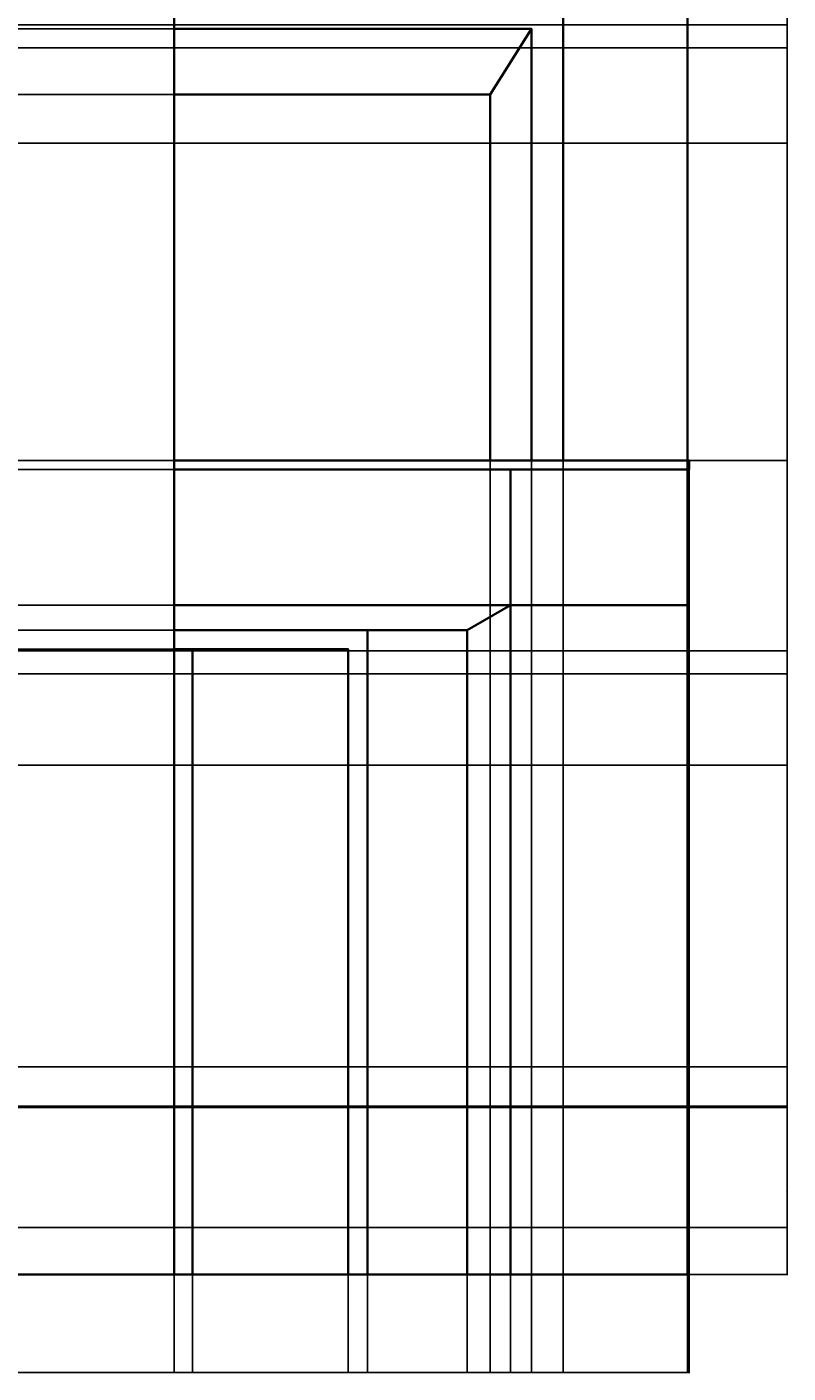
# Model space of a CAD drawing. Units: feet. Extents: x 4092 to 5585, y 725 to 1390.
# Tile 6 of 7: x 5346 to 5585, y 725 to 1146. Entities that reach past the tile are written whole.
import ezdxf

# ---------------------------------------------------------------- set-up
doc = ezdxf.new("R2010")
doc.units = ezdxf.units.FT
doc.layers.add('A-ANNO-DIMS', color=2, linetype='Continuous', lineweight=18)
doc.layers.add('A-ELEV', color=7, linetype='Continuous', lineweight=35)
doc.styles.get("Standard").update_dxf_attribs({"font": 'arial.ttf'})
doc.dimstyles.get("Standard").update_dxf_attribs({"dimtxt": 0.18, "dimasz": 0.18, "dimexe": 0.18, "dimexo": 0.0625, "dimgap": 0.09, "dimtad": 0, "dimtih": 1, "dimtoh": 1, "dimdec": 1, "dimzin": 0, "dimdsep": 46, "dimlunit": 3, "dimtxsty": 'Standard', "dimcen": 0.09, "dimadec": 0, "dimazin": 0, "dimtfac": 1, "dimtdec": 1, "dimtofl": 0, "dimtmove": 0, "dimatfit": 3, "dimfxl": 1, "dimtolj": 1, "dimtzin": 0, "dimarcsym": 0})

# ---------------------------------------------------------------- blocks, each defined once
blk = doc.blocks.new('*D4')
at = {"layer": 'A-ANNO-DIMS', "color": 0, "lineweight": -2, "transparency": 16777216}
for p, q in [((4953.29, 755.89), (4953.29, 725.07)), ((5553.29, 755.89), (5553.29, 725.07)), ((4953.47, 725.25), (5253, 725.25)), ((5553.11, 725.25), (5253.58, 725.25))]:
    blk.add_line(p, q, dxfattribs=at)
at = {"layer": 'A-ANNO-DIMS', "color": 0, "transparency": 16777216}
for points in [[(4953.47, 725.28), (4953.47, 725.22), (4953.29, 725.25)], [(5553.11, 725.28), (5553.11, 725.22), (5553.29, 725.25)]]:
    blk.add_solid(points, dxfattribs=at)
at = {"layer": 'Defpoints', "color": 0, "transparency": 16777216}
for p in [(4953.29, 755.95), (5553.29, 755.95), (5553.29, 725.25)]:
    blk.add_point(p, dxfattribs=at)
at = {"layer": 'A-ANNO-DIMS', "color": 0, "transparency": 16777216, "insert": (5253.29, 725.25), "char_height": 0.18, "attachment_point": 5}
blk.add_mtext('\\A1;600', dxfattribs=at)
blk = doc.blocks.new('*D5')
at = {"layer": 'A-ANNO-DIMS', "color": 0, "lineweight": -2, "transparency": 16777216}
for p, q in [((5264.26, 1358.97), (5584.71, 1358.97)), ((5584.53, 1358.79), (5584.53, 1057.64)), ((5584.53, 756.13), (5584.53, 1057.28)), ((5553.36, 755.95), (5584.71, 755.95))]:
    blk.add_line(p, q, dxfattribs=at)
at = {"layer": 'A-ANNO-DIMS', "color": 0, "transparency": 16777216}
for points in [[(5584.5, 1358.79), (5584.56, 1358.79), (5584.53, 1358.97)], [(5584.5, 756.13), (5584.56, 756.13), (5584.53, 755.95)]]:
    blk.add_solid(points, dxfattribs=at)
at = {"layer": 'Defpoints', "color": 0, "transparency": 16777216}
for p in [(5264.2, 1358.97), (5584.53, 1358.97), (5553.29, 755.95)]:
    blk.add_point(p, dxfattribs=at)
at = {"layer": 'A-ANNO-DIMS', "color": 0, "transparency": 16777216, "insert": (5584.53, 1057.46), "char_height": 0.18, "attachment_point": 5}
blk.add_mtext('\\A1;603', dxfattribs=at)
blk = doc.blocks.new('*D33')
at = {"layer": 'A-ANNO-DIMS', "color": 0, "lineweight": -2, "transparency": 16777216}
for p, q in [((5153.4, 808.21), (5584.71, 808.21)), ((5584.53, 808.03), (5584.53, 782.26)), ((5584.53, 756.13), (5584.53, 781.9)), ((5153.4, 755.95), (5584.71, 755.95))]:
    blk.add_line(p, q, dxfattribs=at)
at = {"layer": 'A-ANNO-DIMS', "color": 0, "transparency": 16777216}
for points in [[(5584.5, 808.03), (5584.56, 808.03), (5584.53, 808.21)], [(5584.5, 756.13), (5584.56, 756.13), (5584.53, 755.95)]]:
    blk.add_solid(points, dxfattribs=at)
at = {"layer": 'Defpoints', "color": 0, "transparency": 16777216}
for p in [(5153.34, 808.21), (5584.53, 808.21), (5153.34, 755.95)]:
    blk.add_point(p, dxfattribs=at)
at = {"layer": 'A-ANNO-DIMS', "color": 0, "transparency": 16777216, "insert": (5584.53, 782.08), "char_height": 0.18, "attachment_point": 5}
blk.add_mtext('\\A1;52.27', dxfattribs=at)
blk = doc.blocks.new('*D34')
at = {"layer": 'A-ANNO-DIMS', "color": 0, "lineweight": -2, "transparency": 16777216}
for p, q in [((5153.4, 915.42), (5584.71, 915.42)), ((5584.53, 915.24), (5584.53, 862)), ((5584.53, 808.39), (5584.53, 861.63)), ((5153.4, 808.21), (5584.71, 808.21))]:
    blk.add_line(p, q, dxfattribs=at)
at = {"layer": 'A-ANNO-DIMS', "color": 0, "transparency": 16777216}
for points in [[(5584.5, 915.24), (5584.56, 915.24), (5584.53, 915.42)], [(5584.5, 808.39), (5584.56, 808.39), (5584.53, 808.21)]]:
    blk.add_solid(points, dxfattribs=at)
at = {"layer": 'Defpoints', "color": 0, "transparency": 16777216}
for p in [(5153.34, 915.42), (5584.53, 915.42), (5153.34, 808.21)]:
    blk.add_point(p, dxfattribs=at)
at = {"layer": 'A-ANNO-DIMS', "color": 0, "transparency": 16777216, "insert": (5584.53, 861.82), "char_height": 0.18, "attachment_point": 5}
blk.add_mtext('\\A1;107.2', dxfattribs=at)
blk = doc.blocks.new('*D35')
at = {"layer": 'A-ANNO-DIMS', "color": 0, "lineweight": -2, "transparency": 16777216}
for p, q in [((5153.4, 944.01), (5584.71, 944.01)), ((5584.53, 943.83), (5584.53, 929.9)), ((5584.53, 915.6), (5584.53, 929.53)), ((5153.4, 915.42), (5584.71, 915.42))]:
    blk.add_line(p, q, dxfattribs=at)
at = {"layer": 'A-ANNO-DIMS', "color": 0, "transparency": 16777216}
for points in [[(5584.5, 943.83), (5584.56, 943.83), (5584.53, 944.01)], [(5584.5, 915.6), (5584.56, 915.6), (5584.53, 915.42)]]:
    blk.add_solid(points, dxfattribs=at)
at = {"layer": 'Defpoints', "color": 0, "transparency": 16777216}
for p in [(5153.34, 944.01), (5584.53, 944.01), (5153.34, 915.42)]:
    blk.add_point(p, dxfattribs=at)
at = {"layer": 'A-ANNO-DIMS', "color": 0, "transparency": 16777216, "insert": (5584.53, 929.71), "char_height": 0.18, "attachment_point": 5}
blk.add_mtext('\\A1;28.59', dxfattribs=at)
blk = doc.blocks.new('*D36')
at = {"layer": 'A-ANNO-DIMS', "color": 0, "lineweight": -2, "transparency": 16777216}
for p, q in [((5160.6, 951.2), (5584.71, 951.2)), ((5584.53, 951.02), (5584.53, 947.79)), ((5153.4, 944.01), (5584.71, 944.01)), ((5584.53, 944.19), (5584.53, 947.42))]:
    blk.add_line(p, q, dxfattribs=at)
at = {"layer": 'A-ANNO-DIMS', "color": 0, "transparency": 16777216}
for points in [[(5584.5, 951.02), (5584.56, 951.02), (5584.53, 951.2)], [(5584.5, 944.19), (5584.56, 944.19), (5584.53, 944.01)]]:
    blk.add_solid(points, dxfattribs=at)
at = {"layer": 'Defpoints', "color": 0, "transparency": 16777216}
for p in [(5160.53, 951.2), (5584.53, 951.2), (5153.34, 944.01)]:
    blk.add_point(p, dxfattribs=at)
at = {"layer": 'A-ANNO-DIMS', "color": 0, "transparency": 16777216, "insert": (5584.53, 947.61), "char_height": 0.18, "attachment_point": 5}
blk.add_mtext('\\A1;7.194', dxfattribs=at)
blk = doc.blocks.new('*D37')
at = {"layer": 'A-ANNO-DIMS', "color": 0, "lineweight": -2, "transparency": 16777216}
for p, q in [((5094.36, 770.68), (5584.71, 770.68)), ((5584.53, 770.5), (5584.53, 763.5)), ((5584.53, 756.13), (5584.53, 763.13)), ((5057.45, 755.95), (5584.71, 755.95))]:
    blk.add_line(p, q, dxfattribs=at)
at = {"layer": 'A-ANNO-DIMS', "color": 0, "transparency": 16777216}
for points in [[(5584.5, 770.5), (5584.56, 770.5), (5584.53, 770.68)], [(5584.5, 756.13), (5584.56, 756.13), (5584.53, 755.95)]]:
    blk.add_solid(points, dxfattribs=at)
at = {"layer": 'Defpoints', "color": 0, "transparency": 16777216}
for p in [(5094.3, 770.68), (5584.53, 770.68), (5057.39, 755.95)]:
    blk.add_point(p, dxfattribs=at)
at = {"layer": 'A-ANNO-DIMS', "color": 0, "transparency": 16777216, "insert": (5584.53, 763.31), "char_height": 0.18, "attachment_point": 5}
blk.add_mtext('\\A1;14.73', dxfattribs=at)
blk = doc.blocks.new('*D38')
at = {"layer": 'A-ANNO-DIMS', "color": 0, "lineweight": -2, "transparency": 16777216}
for p, q in [((5094.36, 808.65), (5584.71, 808.65)), ((5584.53, 808.47), (5584.53, 789.85)), ((5584.53, 770.86), (5584.53, 789.48)), ((5094.36, 770.68), (5584.71, 770.68))]:
    blk.add_line(p, q, dxfattribs=at)
at = {"layer": 'A-ANNO-DIMS', "color": 0, "transparency": 16777216}
for points in [[(5584.5, 808.47), (5584.56, 808.47), (5584.53, 808.65)], [(5584.5, 770.86), (5584.56, 770.86), (5584.53, 770.68)]]:
    blk.add_solid(points, dxfattribs=at)
at = {"layer": 'Defpoints', "color": 0, "transparency": 16777216}
for p in [(5094.3, 808.65), (5584.53, 808.65), (5094.3, 770.68)]:
    blk.add_point(p, dxfattribs=at)
at = {"layer": 'A-ANNO-DIMS', "color": 0, "transparency": 16777216, "insert": (5584.53, 789.67), "char_height": 0.18, "attachment_point": 5}
blk.add_mtext('\\A1;37.97', dxfattribs=at)
blk = doc.blocks.new('*D57')
at = {"layer": 'A-ANNO-DIMS', "color": 0, "lineweight": -2, "transparency": 16777216}
for p, q in [((5153.4, 1110.12), (5584.71, 1110.12)), ((5584.53, 1109.94), (5584.53, 1060.64)), ((5584.53, 1010.97), (5584.53, 1060.27)), ((5185.39, 1010.79), (5584.71, 1010.79))]:
    blk.add_line(p, q, dxfattribs=at)
at = {"layer": 'A-ANNO-DIMS', "color": 0, "transparency": 16777216}
for points in [[(5584.5, 1109.94), (5584.56, 1109.94), (5584.53, 1110.12)], [(5584.5, 1010.97), (5584.56, 1010.97), (5584.53, 1010.79)]]:
    blk.add_solid(points, dxfattribs=at)
at = {"layer": 'Defpoints', "color": 0, "transparency": 16777216}
for p in [(5153.34, 1110.12), (5584.53, 1110.12), (5185.33, 1010.79)]:
    blk.add_point(p, dxfattribs=at)
at = {"layer": 'A-ANNO-DIMS', "color": 0, "transparency": 16777216, "insert": (5584.53, 1060.45), "char_height": 0.18, "attachment_point": 5}
blk.add_mtext('\\A1;99.33', dxfattribs=at)
blk = doc.blocks.new('*D58')
at = {"layer": 'A-ANNO-DIMS', "color": 0, "lineweight": -2, "transparency": 16777216}
for p, q in [((5153.4, 1139.88), (5584.71, 1139.88)), ((5584.53, 1139.7), (5584.53, 1125.18)), ((5584.53, 1110.3), (5584.53, 1124.82)), ((5153.4, 1110.12), (5584.71, 1110.12))]:
    blk.add_line(p, q, dxfattribs=at)
at = {"layer": 'A-ANNO-DIMS', "color": 0, "transparency": 16777216}
for points in [[(5584.5, 1139.7), (5584.56, 1139.7), (5584.53, 1139.88)], [(5584.5, 1110.3), (5584.56, 1110.3), (5584.53, 1110.12)]]:
    blk.add_solid(points, dxfattribs=at)
at = {"layer": 'Defpoints', "color": 0, "transparency": 16777216}
for p in [(5153.34, 1139.88), (5584.53, 1139.88), (5153.34, 1110.12)]:
    blk.add_point(p, dxfattribs=at)
at = {"layer": 'A-ANNO-DIMS', "color": 0, "transparency": 16777216, "insert": (5584.53, 1125), "char_height": 0.18, "attachment_point": 5}
blk.add_mtext('\\A1;29.76', dxfattribs=at)
blk = doc.blocks.new('*D59')
at = {"layer": 'A-ANNO-DIMS', "color": 0, "lineweight": -2, "transparency": 16777216}
for p, q in [((5185.39, 1147.07), (5584.71, 1147.07)), ((5584.53, 1146.89), (5584.53, 1143.66)), ((5584.53, 1140.06), (5584.53, 1143.3)), ((5153.4, 1139.88), (5584.71, 1139.88))]:
    blk.add_line(p, q, dxfattribs=at)
at = {"layer": 'A-ANNO-DIMS', "color": 0, "transparency": 16777216}
for points in [[(5584.5, 1146.89), (5584.56, 1146.89), (5584.53, 1147.07)], [(5584.5, 1140.06), (5584.56, 1140.06), (5584.53, 1139.88)]]:
    blk.add_solid(points, dxfattribs=at)
at = {"layer": 'Defpoints', "color": 0, "transparency": 16777216}
for p in [(5185.33, 1147.07), (5584.53, 1147.07), (5153.34, 1139.88)]:
    blk.add_point(p, dxfattribs=at)
at = {"layer": 'A-ANNO-DIMS', "color": 0, "transparency": 16777216, "insert": (5584.53, 1143.48), "char_height": 0.18, "attachment_point": 5}
blk.add_mtext('\\A1;7.194', dxfattribs=at)
blk = doc.blocks.new('*D64')
at = {"layer": 'A-ANNO-DIMS', "color": 0, "lineweight": -2, "transparency": 16777216}
for p, q in [((5285.79, 755.89), (5285.79, 725.07)), ((5392.55, 755.89), (5392.55, 725.07)), ((5285.97, 725.25), (5338.72, 725.25)), ((5392.37, 725.25), (5339.63, 725.25))]:
    blk.add_line(p, q, dxfattribs=at)
at = {"layer": 'A-ANNO-DIMS', "color": 0, "transparency": 16777216}
for points in [[(5285.97, 725.28), (5285.97, 725.22), (5285.79, 725.25)], [(5392.37, 725.28), (5392.37, 725.22), (5392.55, 725.25)]]:
    blk.add_solid(points, dxfattribs=at)
at = {"layer": 'Defpoints', "color": 0, "transparency": 16777216}
for p in [(5285.79, 755.95), (5392.55, 755.95), (5392.55, 725.25)]:
    blk.add_point(p, dxfattribs=at)
at = {"layer": 'A-ANNO-DIMS', "color": 0, "transparency": 16777216, "insert": (5339.17, 725.25), "char_height": 0.18, "attachment_point": 5}
blk.add_mtext('\\A1;106.76', dxfattribs=at)
blk = doc.blocks.new('*D65')
at = {"layer": 'A-ANNO-DIMS', "color": 0, "lineweight": -2, "transparency": 16777216}
for p, q in [((5392.55, 755.89), (5392.55, 725.07)), ((5398.25, 755.89), (5398.25, 725.07)), ((5392.73, 725.25), (5395.01, 725.25)), ((5398.07, 725.25), (5395.79, 725.25))]:
    blk.add_line(p, q, dxfattribs=at)
at = {"layer": 'A-ANNO-DIMS', "color": 0, "transparency": 16777216}
for points in [[(5392.73, 725.28), (5392.73, 725.22), (5392.55, 725.25)], [(5398.07, 725.28), (5398.07, 725.22), (5398.25, 725.25)]]:
    blk.add_solid(points, dxfattribs=at)
at = {"layer": 'Defpoints', "color": 0, "transparency": 16777216}
for p in [(5392.55, 755.95), (5398.25, 755.95), (5398.25, 725.25)]:
    blk.add_point(p, dxfattribs=at)
at = {"layer": 'A-ANNO-DIMS', "color": 0, "transparency": 16777216, "insert": (5395.4, 725.25), "char_height": 0.18, "attachment_point": 5}
blk.add_mtext('\\A1;5.694', dxfattribs=at)
blk = doc.blocks.new('*D66')
at = {"layer": 'A-ANNO-DIMS', "color": 0, "lineweight": -2, "transparency": 16777216}
for p, q in [((5398.25, 755.89), (5398.25, 725.07)), ((5447.06, 755.89), (5447.06, 725.07)), ((5398.43, 725.25), (5422.27, 725.25)), ((5446.88, 725.25), (5423.03, 725.25))]:
    blk.add_line(p, q, dxfattribs=at)
at = {"layer": 'A-ANNO-DIMS', "color": 0, "transparency": 16777216}
for points in [[(5398.43, 725.28), (5398.43, 725.22), (5398.25, 725.25)], [(5446.88, 725.28), (5446.88, 725.22), (5447.06, 725.25)]]:
    blk.add_solid(points, dxfattribs=at)
at = {"layer": 'Defpoints', "color": 0, "transparency": 16777216}
for p in [(5398.25, 755.95), (5447.06, 755.95), (5447.06, 725.25)]:
    blk.add_point(p, dxfattribs=at)
at = {"layer": 'A-ANNO-DIMS', "color": 0, "transparency": 16777216, "insert": (5422.65, 725.25), "char_height": 0.18, "attachment_point": 5}
blk.add_mtext('\\A1;48.81', dxfattribs=at)
blk = doc.blocks.new('*D67')
at = {"layer": 'A-ANNO-DIMS', "color": 0, "lineweight": -2, "transparency": 16777216}
for p, q in [((5447.06, 755.89), (5447.06, 725.07)), ((5453.06, 755.89), (5453.06, 725.07)), ((5447.24, 725.25), (5449.91, 725.25)), ((5452.88, 725.25), (5450.21, 725.25))]:
    blk.add_line(p, q, dxfattribs=at)
at = {"layer": 'A-ANNO-DIMS', "color": 0, "transparency": 16777216}
for points in [[(5447.24, 725.28), (5447.24, 725.22), (5447.06, 725.25)], [(5452.88, 725.28), (5452.88, 725.22), (5453.06, 725.25)]]:
    blk.add_solid(points, dxfattribs=at)
at = {"layer": 'Defpoints', "color": 0, "transparency": 16777216}
for p in [(5447.06, 755.95), (5453.06, 755.95), (5453.06, 725.25)]:
    blk.add_point(p, dxfattribs=at)
at = {"layer": 'A-ANNO-DIMS', "color": 0, "transparency": 16777216, "insert": (5450.06, 725.25), "char_height": 0.18, "attachment_point": 5}
blk.add_mtext('\\A1;6', dxfattribs=at)
blk = doc.blocks.new('*D68')
at = {"layer": 'A-ANNO-DIMS', "color": 0, "lineweight": -2, "transparency": 16777216}
for p, q in [((5453.06, 755.89), (5453.06, 725.07)), ((5484.32, 755.89), (5484.32, 725.07)), ((5453.24, 725.25), (5468.29, 725.25)), ((5484.14, 725.25), (5469.08, 725.25))]:
    blk.add_line(p, q, dxfattribs=at)
at = {"layer": 'A-ANNO-DIMS', "color": 0, "transparency": 16777216}
for points in [[(5453.24, 725.28), (5453.24, 725.22), (5453.06, 725.25)], [(5484.14, 725.28), (5484.14, 725.22), (5484.32, 725.25)]]:
    blk.add_solid(points, dxfattribs=at)
at = {"layer": 'Defpoints', "color": 0, "transparency": 16777216}
for p in [(5453.06, 755.95), (5484.32, 755.95), (5484.32, 725.25)]:
    blk.add_point(p, dxfattribs=at)
at = {"layer": 'A-ANNO-DIMS', "color": 0, "transparency": 16777216, "insert": (5468.69, 725.25), "char_height": 0.18, "attachment_point": 5}
blk.add_mtext('\\A1;31.26', dxfattribs=at)
blk = doc.blocks.new('*D69')
at = {"layer": 'A-ANNO-DIMS', "color": 0, "lineweight": -2, "transparency": 16777216}
for p, q in [((5484.32, 755.89), (5484.32, 725.07)), ((5497.93, 755.89), (5497.93, 725.07)), ((5484.5, 725.25), (5490.76, 725.25)), ((5497.75, 725.25), (5491.49, 725.25))]:
    blk.add_line(p, q, dxfattribs=at)
at = {"layer": 'A-ANNO-DIMS', "color": 0, "transparency": 16777216}
for points in [[(5484.5, 725.28), (5484.5, 725.22), (5484.32, 725.25)], [(5497.75, 725.28), (5497.75, 725.22), (5497.93, 725.25)]]:
    blk.add_solid(points, dxfattribs=at)
at = {"layer": 'Defpoints', "color": 0, "transparency": 16777216}
for p in [(5484.32, 755.95), (5497.93, 755.95), (5497.93, 725.25)]:
    blk.add_point(p, dxfattribs=at)
at = {"layer": 'A-ANNO-DIMS', "color": 0, "transparency": 16777216, "insert": (5491.12, 725.25), "char_height": 0.18, "attachment_point": 5}
blk.add_mtext('\\A1;13.61', dxfattribs=at)
blk = doc.blocks.new('*D70')
at = {"layer": 'A-ANNO-DIMS', "color": 0, "lineweight": -2, "transparency": 16777216}
for p, q in [((5497.93, 755.89), (5497.93, 725.07)), ((5553.29, 755.89), (5553.29, 725.07)), ((5498.11, 725.25), (5525.22, 725.25)), ((5553.11, 725.25), (5526, 725.25))]:
    blk.add_line(p, q, dxfattribs=at)
at = {"layer": 'A-ANNO-DIMS', "color": 0, "transparency": 16777216}
for points in [[(5498.11, 725.28), (5498.11, 725.22), (5497.93, 725.25)], [(5553.11, 725.28), (5553.11, 725.22), (5553.29, 725.25)]]:
    blk.add_solid(points, dxfattribs=at)
at = {"layer": 'Defpoints', "color": 0, "transparency": 16777216}
for p in [(5497.93, 755.95), (5553.29, 755.95), (5553.29, 725.25)]:
    blk.add_point(p, dxfattribs=at)
at = {"layer": 'A-ANNO-DIMS', "color": 0, "transparency": 16777216, "insert": (5525.61, 725.25), "char_height": 0.18, "attachment_point": 5}
blk.add_mtext('\\A1;55.36', dxfattribs=at)
blk = doc.blocks.new('*D73')
at = {"layer": 'A-ANNO-DIMS', "color": 0, "lineweight": -2, "transparency": 16777216}
for p, q in [((5339.81, 820.92), (5584.71, 820.92)), ((5584.53, 820.74), (5584.53, 788.62)), ((5584.53, 756.13), (5584.53, 788.25)), ((5285.85, 755.95), (5584.71, 755.95))]:
    blk.add_line(p, q, dxfattribs=at)
at = {"layer": 'A-ANNO-DIMS', "color": 0, "transparency": 16777216}
for points in [[(5584.5, 820.74), (5584.56, 820.74), (5584.53, 820.92)], [(5584.5, 756.13), (5584.56, 756.13), (5584.53, 755.95)]]:
    blk.add_solid(points, dxfattribs=at)
at = {"layer": 'Defpoints', "color": 0, "transparency": 16777216}
for p in [(5339.75, 820.92), (5584.53, 820.92), (5285.79, 755.95)]:
    blk.add_point(p, dxfattribs=at)
at = {"layer": 'A-ANNO-DIMS', "color": 0, "transparency": 16777216, "insert": (5584.53, 788.43), "char_height": 0.18, "attachment_point": 5}
blk.add_mtext('\\A1;64.97', dxfattribs=at)
blk = doc.blocks.new('*D75')
at = {"layer": 'A-ANNO-DIMS', "color": 0, "lineweight": -2, "transparency": 16777216}
for p, q in [((5392.49, 951.65), (4921.27, 951.65)), ((4921.45, 951.47), (4921.45, 853.98)), ((4921.45, 756.13), (4921.45, 853.62)), ((5392.49, 755.95), (4921.27, 755.95))]:
    blk.add_line(p, q, dxfattribs=at)
at = {"layer": 'A-ANNO-DIMS', "color": 0, "transparency": 16777216}
for points in [[(4921.42, 951.47), (4921.48, 951.47), (4921.45, 951.65)], [(4921.42, 756.13), (4921.48, 756.13), (4921.45, 755.95)]]:
    blk.add_solid(points, dxfattribs=at)
at = {"layer": 'Defpoints', "color": 0, "transparency": 16777216}
for p in [(4921.45, 951.65), (5392.55, 951.65), (5392.55, 755.95)]:
    blk.add_point(p, dxfattribs=at)
at = {"layer": 'A-ANNO-DIMS', "color": 0, "transparency": 16777216, "insert": (4921.45, 853.8), "char_height": 0.18, "attachment_point": 5}
blk.add_mtext('\\A1;195.7', dxfattribs=at)
blk = doc.blocks.new('*D76')
at = {"layer": 'A-ANNO-DIMS', "color": 0, "lineweight": -2, "transparency": 16777216}
for p, q in [((5392.49, 957.65), (4921.27, 957.65)), ((4921.45, 957.47), (4921.45, 954.83)), ((4921.45, 951.83), (4921.45, 954.46)), ((5392.49, 951.65), (4921.27, 951.65))]:
    blk.add_line(p, q, dxfattribs=at)
at = {"layer": 'A-ANNO-DIMS', "color": 0, "transparency": 16777216}
for points in [[(4921.42, 957.47), (4921.48, 957.47), (4921.45, 957.65)], [(4921.42, 951.83), (4921.48, 951.83), (4921.45, 951.65)]]:
    blk.add_solid(points, dxfattribs=at)
at = {"layer": 'Defpoints', "color": 0, "transparency": 16777216}
for p in [(4921.45, 957.65), (5392.55, 957.65), (5392.55, 951.65)]:
    blk.add_point(p, dxfattribs=at)
at = {"layer": 'A-ANNO-DIMS', "color": 0, "transparency": 16777216, "insert": (4921.45, 954.65), "char_height": 0.18, "attachment_point": 5}
blk.add_mtext('\\A1;6', dxfattribs=at)
blk = doc.blocks.new('*D77')
at = {"layer": 'A-ANNO-DIMS', "color": 0, "lineweight": -2, "transparency": 16777216}
for p, q in [((5392.49, 965.48), (4921.27, 965.48)), ((4921.45, 965.3), (4921.45, 961.74)), ((4921.45, 957.83), (4921.45, 961.38)), ((5392.49, 957.65), (4921.27, 957.65))]:
    blk.add_line(p, q, dxfattribs=at)
at = {"layer": 'A-ANNO-DIMS', "color": 0, "transparency": 16777216}
for points in [[(4921.42, 965.3), (4921.48, 965.3), (4921.45, 965.48)], [(4921.42, 957.83), (4921.48, 957.83), (4921.45, 957.65)]]:
    blk.add_solid(points, dxfattribs=at)
at = {"layer": 'Defpoints', "color": 0, "transparency": 16777216}
for p in [(4921.45, 965.48), (5392.55, 965.48), (5392.55, 957.65)]:
    blk.add_point(p, dxfattribs=at)
at = {"layer": 'A-ANNO-DIMS', "color": 0, "transparency": 16777216, "insert": (4921.45, 961.56), "char_height": 0.18, "attachment_point": 5}
blk.add_mtext('\\A1;7.833', dxfattribs=at)
blk = doc.blocks.new('*D78')
at = {"layer": 'A-ANNO-DIMS', "color": 0, "lineweight": -2, "transparency": 16777216}
for p, q in [((5392.49, 1007.95), (4921.27, 1007.95)), ((4921.45, 1007.77), (4921.45, 986.89)), ((4921.45, 965.66), (4921.45, 986.53)), ((5392.49, 965.48), (4921.27, 965.48))]:
    blk.add_line(p, q, dxfattribs=at)
at = {"layer": 'A-ANNO-DIMS', "color": 0, "transparency": 16777216}
for points in [[(4921.42, 1007.77), (4921.48, 1007.77), (4921.45, 1007.95)], [(4921.42, 965.66), (4921.48, 965.66), (4921.45, 965.48)]]:
    blk.add_solid(points, dxfattribs=at)
at = {"layer": 'Defpoints', "color": 0, "transparency": 16777216}
for p in [(4921.45, 1007.95), (5392.55, 1007.95), (5392.55, 965.48)]:
    blk.add_point(p, dxfattribs=at)
at = {"layer": 'A-ANNO-DIMS', "color": 0, "transparency": 16777216, "insert": (4921.45, 986.71), "char_height": 0.18, "attachment_point": 5}
blk.add_mtext('\\A1;42.47', dxfattribs=at)
blk = doc.blocks.new('*D79')
at = {"layer": 'A-ANNO-DIMS', "color": 0, "lineweight": -2, "transparency": 16777216}
for p, q in [((5392.49, 1125.34), (4921.27, 1125.34)), ((4921.45, 1125.16), (4921.45, 1068.25)), ((4921.45, 1010.97), (4921.45, 1067.88)), ((5392.49, 1010.79), (4921.27, 1010.79))]:
    blk.add_line(p, q, dxfattribs=at)
at = {"layer": 'A-ANNO-DIMS', "color": 0, "transparency": 16777216}
for points in [[(4921.42, 1125.16), (4921.48, 1125.16), (4921.45, 1125.34)], [(4921.42, 1010.97), (4921.48, 1010.97), (4921.45, 1010.79)]]:
    blk.add_solid(points, dxfattribs=at)
at = {"layer": 'Defpoints', "color": 0, "transparency": 16777216}
for p in [(4921.45, 1125.34), (5392.55, 1125.34), (5392.55, 1010.79)]:
    blk.add_point(p, dxfattribs=at)
at = {"layer": 'A-ANNO-DIMS', "color": 0, "transparency": 16777216, "insert": (4921.45, 1068.07), "char_height": 0.18, "attachment_point": 5}
blk.add_mtext('\\A1;114.55', dxfattribs=at)
blk = doc.blocks.new('*D80')
at = {"layer": 'A-ANNO-DIMS', "color": 0, "lineweight": -2, "transparency": 16777216}
for p, q in [((5392.49, 1145.86), (4921.27, 1145.86)), ((4921.45, 1145.68), (4921.45, 1135.78)), ((4921.45, 1125.52), (4921.45, 1135.42)), ((5392.49, 1125.34), (4921.27, 1125.34))]:
    blk.add_line(p, q, dxfattribs=at)
at = {"layer": 'A-ANNO-DIMS', "color": 0, "transparency": 16777216}
for points in [[(4921.42, 1145.68), (4921.48, 1145.68), (4921.45, 1145.86)], [(4921.42, 1125.52), (4921.48, 1125.52), (4921.45, 1125.34)]]:
    blk.add_solid(points, dxfattribs=at)
at = {"layer": 'Defpoints', "color": 0, "transparency": 16777216}
for p in [(4921.45, 1145.86), (5392.55, 1145.86), (5392.55, 1125.34)]:
    blk.add_point(p, dxfattribs=at)
at = {"layer": 'A-ANNO-DIMS', "color": 0, "transparency": 16777216, "insert": (4921.45, 1135.6), "char_height": 0.18, "attachment_point": 5}
blk.add_mtext('\\A1;20.52', dxfattribs=at)
blk = doc.blocks.new('*D81')
at = {"layer": 'A-ANNO-DIMS', "color": 0, "lineweight": -2, "transparency": 16777216}
for p, q in [((5392.49, 1171.51), (4921.27, 1171.51)), ((4921.45, 1171.33), (4921.45, 1158.87)), ((4921.45, 1146.04), (4921.45, 1158.5)), ((5392.49, 1145.86), (4921.27, 1145.86))]:
    blk.add_line(p, q, dxfattribs=at)
at = {"layer": 'A-ANNO-DIMS', "color": 0, "transparency": 16777216}
for points in [[(4921.42, 1171.33), (4921.48, 1171.33), (4921.45, 1171.51)], [(4921.42, 1146.04), (4921.48, 1146.04), (4921.45, 1145.86)]]:
    blk.add_solid(points, dxfattribs=at)
at = {"layer": 'Defpoints', "color": 0, "transparency": 16777216}
for p in [(4921.45, 1171.51), (5392.55, 1171.51), (5392.55, 1145.86)]:
    blk.add_point(p, dxfattribs=at)
at = {"layer": 'A-ANNO-DIMS', "color": 0, "transparency": 16777216, "insert": (4921.45, 1158.69), "char_height": 0.18, "attachment_point": 5}
blk.add_mtext('\\A1;25.65', dxfattribs=at)
blk = doc.blocks.new('*D88')
at = {"layer": 'A-ANNO-DIMS', "color": 0, "lineweight": -2, "transparency": 16777216}
for p, q in [((5392.55, 1010.73), (5392.55, 725.07)), ((5491.48, 1010.73), (5491.48, 725.07)), ((5392.73, 725.25), (5441.62, 725.25)), ((5491.3, 725.25), (5442.41, 725.25))]:
    blk.add_line(p, q, dxfattribs=at)
at = {"layer": 'A-ANNO-DIMS', "color": 0, "transparency": 16777216}
for points in [[(5392.73, 725.28), (5392.73, 725.22), (5392.55, 725.25)], [(5491.3, 725.28), (5491.3, 725.22), (5491.48, 725.25)]]:
    blk.add_solid(points, dxfattribs=at)
at = {"layer": 'Defpoints', "color": 0, "transparency": 16777216}
for p in [(5392.55, 1010.79), (5491.48, 1010.79), (5491.48, 725.25)]:
    blk.add_point(p, dxfattribs=at)
at = {"layer": 'A-ANNO-DIMS', "color": 0, "transparency": 16777216, "insert": (5442.01, 725.25), "char_height": 0.18, "attachment_point": 5}
blk.add_mtext('\\A1;98.93', dxfattribs=at)
blk = doc.blocks.new('*D89')
at = {"layer": 'A-ANNO-DIMS', "color": 0, "lineweight": -2, "transparency": 16777216}
for p, q in [((5491.48, 1010.73), (5491.48, 725.07)), ((5504.46, 1010.73), (5504.46, 725.07)), ((5491.66, 725.25), (5497.52, 725.25)), ((5504.28, 725.25), (5498.43, 725.25))]:
    blk.add_line(p, q, dxfattribs=at)
at = {"layer": 'A-ANNO-DIMS', "color": 0, "transparency": 16777216}
for points in [[(5491.66, 725.28), (5491.66, 725.22), (5491.48, 725.25)], [(5504.28, 725.28), (5504.28, 725.22), (5504.46, 725.25)]]:
    blk.add_solid(points, dxfattribs=at)
at = {"layer": 'Defpoints', "color": 0, "transparency": 16777216}
for p in [(5491.48, 1010.79), (5504.46, 1010.79), (5504.46, 725.25)]:
    blk.add_point(p, dxfattribs=at)
at = {"layer": 'A-ANNO-DIMS', "color": 0, "transparency": 16777216, "insert": (5497.97, 725.25), "char_height": 0.18, "attachment_point": 5}
blk.add_mtext('\\A1;12.986', dxfattribs=at)
blk = doc.blocks.new('*D90')
at = {"layer": 'A-ANNO-DIMS', "color": 0, "lineweight": -2, "transparency": 16777216}
for p, q in [((5504.46, 1010.73), (5504.46, 725.07)), ((5514.33, 1010.73), (5514.33, 725.07)), ((5504.64, 725.25), (5509, 725.25)), ((5514.15, 725.25), (5509.79, 725.25))]:
    blk.add_line(p, q, dxfattribs=at)
at = {"layer": 'A-ANNO-DIMS', "color": 0, "transparency": 16777216}
for points in [[(5504.64, 725.28), (5504.64, 725.22), (5504.46, 725.25)], [(5514.15, 725.28), (5514.15, 725.22), (5514.33, 725.25)]]:
    blk.add_solid(points, dxfattribs=at)
at = {"layer": 'Defpoints', "color": 0, "transparency": 16777216}
for p in [(5504.46, 1010.79), (5514.33, 1010.79), (5514.33, 725.25)]:
    blk.add_point(p, dxfattribs=at)
at = {"layer": 'A-ANNO-DIMS', "color": 0, "transparency": 16777216, "insert": (5509.4, 725.25), "char_height": 0.18, "attachment_point": 5}
blk.add_mtext('\\A1;9.867', dxfattribs=at)
blk = doc.blocks.new('*D91')
at = {"layer": 'A-ANNO-DIMS', "color": 0, "lineweight": -2, "transparency": 16777216}
for p, q in [((5514.33, 1010.73), (5514.33, 725.07)), ((5553.83, 1010.73), (5553.83, 725.07)), ((5514.51, 725.25), (5533.76, 725.25)), ((5553.65, 725.25), (5534.41, 725.25))]:
    blk.add_line(p, q, dxfattribs=at)
at = {"layer": 'A-ANNO-DIMS', "color": 0, "transparency": 16777216}
for points in [[(5514.51, 725.28), (5514.51, 725.22), (5514.33, 725.25)], [(5553.65, 725.28), (5553.65, 725.22), (5553.83, 725.25)]]:
    blk.add_solid(points, dxfattribs=at)
at = {"layer": 'Defpoints', "color": 0, "transparency": 16777216}
for p in [(5514.33, 1010.79), (5553.83, 1010.79), (5553.83, 725.25)]:
    blk.add_point(p, dxfattribs=at)
at = {"layer": 'A-ANNO-DIMS', "color": 0, "transparency": 16777216, "insert": (5534.08, 725.25), "char_height": 0.18, "attachment_point": 5}
blk.add_mtext('\\A1;39.5', dxfattribs=at)

msp = doc.modelspace()

# ---------------------------------------------------------------- linework, layer by layer
at = {"layer": 'A-ELEV'}
for p, q in [((5553.293, 755.9488), (5553.293, 1229.2703)), ((5504.4634, 1145.8611), (5491.4775, 1125.3426)), ((5497.9281, 965.4789), (5484.3189, 957.6463)), ((5484.3189, 957.6463), (5392.5521, 957.6463)), ((5484.3189, 957.6463), (5484.3189, 755.9488)), ((4953.293, 755.9488), (5553.293, 755.9488))]:
    msp.add_line(p, q, dxfattribs=at)
for points in [[(5392.5521, 755.9488), (5285.7915, 755.9488), (5285.7915, 1305.7746), (5392.5521, 1305.7746)], [(5392.5521, 1010.7906), (5553.8322, 1010.7906), (5553.8322, 1007.9488), (5392.5521, 1007.9488)], [(5392.5521, 1007.9488), (5553.293, 1007.9488), (5553.293, 965.4789), (5392.5521, 965.4789)], [(5553.293, 755.9488), (5497.9281, 755.9488), (5497.9281, 1007.9488), (5553.293, 1007.9488)], [(5392.5521, 957.6463), (5453.0572, 957.6463), (5453.0572, 755.9488), (5392.5521, 755.9488)], [(5392.5521, 951.6463), (5398.2462, 951.6463), (5398.2462, 755.9488), (5392.5521, 755.9488)]]:
    msp.add_lwpolyline(points, close=True, dxfattribs=at)
for points in [[(5514.3304, 1171.511), (5514.3304, 1010.7906), (5392.5521, 1010.7906), (5392.5521, 1125.3426)], [(5491.4775, 1010.7906), (5504.4634, 1010.7906), (5504.4634, 1145.8611), (5392.5521, 1145.8611)], [(5491.4775, 1010.7906), (5491.4775, 1125.3426), (5392.5521, 1125.3426)], [(5392.5521, 951.6463), (5447.0572, 951.6463), (5447.0572, 755.9488)]]:
    msp.add_lwpolyline(points, dxfattribs=at)

# ---------------------------------------------------------------- dimensions: what is measured, and where the dimension line sits
at = {"layer": 'A-ANNO-DIMS'}
for base, p1, p2, override, picture, middle in [((5584.5322, 1358.9731), (5553.293, 755.9488), (5264.1979, 1358.9731), {"dimdec": 0, "dimlfac": 1, "dimrnd": 0, "dimzin": 0, "dimdsep": 46, "dimlunit": 2}, '*D5', (5584.5322, 1057.461)), ((4921.4517, 1171.511), (5392.5521, 1145.8611), (5392.5521, 1171.511), {"dimdec": 2, "dimlfac": 1, "dimrnd": 0, "dimzin": 0, "dimdsep": 46, "dimlunit": 2}, '*D81', (4921.4517, 1158.6861)), ((5584.5322, 1147.0743), (5153.3388, 1139.8803), (5185.3285, 1147.0743), {"dimdec": 3, "dimlfac": 1, "dimrnd": 0, "dimzin": 0, "dimdsep": 46, "dimlunit": 2}, '*D59', (5584.5322, 1143.4773)), ((4921.4517, 1145.8611), (5392.5521, 1125.3426), (5392.5521, 1145.8611), {"dimdec": 2, "dimlfac": 1, "dimrnd": 0, "dimzin": 0, "dimdsep": 46, "dimlunit": 2}, '*D80', (4921.4517, 1135.6018)), ((5584.5322, 1139.8803), (5153.3388, 1110.119), (5153.3388, 1139.8803), {"dimdec": 2, "dimlfac": 1, "dimrnd": 0, "dimzin": 0, "dimdsep": 46, "dimlunit": 2}, '*D58', (5584.5322, 1124.9996)), ((4921.4517, 1125.3426), (5392.5521, 1010.7906), (5392.5521, 1125.3426), {"dimdec": 2, "dimlfac": 1, "dimrnd": 0, "dimzin": 0, "dimdsep": 46, "dimlunit": 2}, '*D79', (4921.4517, 1068.0666)), ((5584.5322, 1110.119), (5185.3285, 1010.7906), (5153.3388, 1110.119), {"dimdec": 2, "dimlfac": 1, "dimrnd": 0, "dimzin": 0, "dimdsep": 46, "dimlunit": 2}, '*D57', (5584.5322, 1060.4548)), ((4921.4517, 1007.9488), (5392.5521, 965.4789), (5392.5521, 1007.9488), {"dimdec": 2, "dimlfac": 1, "dimrnd": 0, "dimzin": 0, "dimdsep": 46, "dimlunit": 2}, '*D78', (4921.4517, 986.7139)), ((4921.4517, 965.4789), (5392.5521, 957.6463), (5392.5521, 965.4789), {"dimdec": 3, "dimlfac": 1, "dimrnd": 0, "dimzin": 0, "dimdsep": 46, "dimlunit": 2}, '*D77', (4921.4517, 961.5626)), ((4921.4517, 957.6463), (5392.5521, 951.6463), (5392.5521, 957.6463), {"dimdec": 0, "dimlfac": 1, "dimrnd": 0, "dimzin": 0, "dimdsep": 46, "dimlunit": 2}, '*D76', (4921.4517, 954.6463)), ((4921.4517, 951.6463), (5392.5521, 755.9488), (5392.5521, 951.6463), {"dimdec": 1, "dimlfac": 1, "dimrnd": 0, "dimzin": 0, "dimdsep": 46, "dimlunit": 2}, '*D75', (4921.4517, 853.7975)), ((5584.5322, 951.2024), (5153.3388, 944.0084), (5160.5329, 951.2024), {"dimdec": 3, "dimlfac": 1, "dimrnd": 0, "dimzin": 0, "dimdsep": 46, "dimlunit": 2}, '*D36', (5584.5322, 947.6054)), ((5584.5322, 944.0084), (5153.3388, 915.418), (5153.3388, 944.0084), {"dimdec": 2, "dimlfac": 1, "dimrnd": 0, "dimzin": 0, "dimdsep": 46, "dimlunit": 2}, '*D35', (5584.5322, 929.7132)), ((5584.5322, 915.418), (5153.3388, 808.2143), (5153.3388, 915.418), {"dimdec": 1, "dimlfac": 1, "dimrnd": 0, "dimzin": 0, "dimdsep": 46, "dimlunit": 2}, '*D34', (5584.5322, 861.8161)), ((5584.5322, 820.9207), (5285.7915, 755.9488), (5339.7523, 820.9207), {"dimdec": 2, "dimlfac": 1, "dimrnd": 0, "dimzin": 0, "dimdsep": 46, "dimlunit": 2}, '*D73', (5584.5322, 788.4347)), ((5584.5322, 808.6527), (5094.3002, 770.6797), (5094.3002, 808.6527), {"dimdec": 2, "dimlfac": 1, "dimrnd": 0, "dimzin": 0, "dimdsep": 46, "dimlunit": 2}, '*D38', (5584.5322, 789.6662)), ((5584.5322, 808.2143), (5153.3388, 755.9488), (5153.3388, 808.2143), {"dimdec": 2, "dimlfac": 1, "dimrnd": 0, "dimzin": 0, "dimdsep": 46, "dimlunit": 2}, '*D33', (5584.5322, 782.0815)), ((5584.5322, 770.6797), (5057.3906, 755.9488), (5094.3002, 770.6797), {"dimdec": 2, "dimlfac": 1, "dimrnd": 0, "dimzin": 0, "dimdsep": 46, "dimlunit": 2}, '*D37', (5584.5322, 763.3143))]:
    dim = msp.add_linear_dim(base=base, p1=p1, p2=p2, angle=90, dimstyle='Standard', override=override, dxfattribs=at)
    dim.commit()
    dim.dimension.update_dxf_attribs({"geometry": picture, "text_midpoint": middle})
for base, p1, p2, override, picture, middle in [((5491.4775, 725.2488), (5392.5521, 1010.7906), (5491.4775, 1010.7906), {"dimdec": 2, "dimlfac": 1, "dimrnd": 0, "dimzin": 0, "dimdsep": 46, "dimlunit": 2}, '*D88', (5442.0148, 725.2488)), ((5504.4634, 725.2488), (5491.4775, 1010.7906), (5504.4634, 1010.7906), {"dimdec": 3, "dimlfac": 1, "dimrnd": 0, "dimzin": 0, "dimdsep": 46, "dimlunit": 2}, '*D89', (5497.9705, 725.2488)), ((5514.3304, 725.2488), (5504.4634, 1010.7906), (5514.3304, 1010.7906), {"dimdec": 3, "dimlfac": 1, "dimrnd": 0, "dimzin": 0, "dimdsep": 46, "dimlunit": 2}, '*D90', (5509.3969, 725.2488)), ((5553.8322, 725.2488), (5514.3304, 1010.7906), (5553.8322, 1010.7906), {"dimdec": 1, "dimlfac": 1, "dimrnd": 0, "dimzin": 0, "dimdsep": 46, "dimlunit": 2}, '*D91', (5534.0813, 725.2488)), ((5553.293, 725.2488), (4953.293, 755.9488), (5553.293, 755.9488), {"dimdec": 0, "dimlfac": 1, "dimrnd": 0, "dimzin": 0, "dimdsep": 46, "dimlunit": 2}, '*D4', (5253.293, 725.2488)), ((5392.5521, 725.2488), (5285.7915, 755.9488), (5392.5521, 755.9488), {"dimdec": 2, "dimlfac": 1, "dimrnd": 0, "dimzin": 0, "dimdsep": 46, "dimlunit": 2}, '*D64', (5339.1718, 725.2488)), ((5398.2462, 725.2488), (5392.5521, 755.9488), (5398.2462, 755.9488), {"dimdec": 3, "dimlfac": 1, "dimrnd": 0, "dimzin": 0, "dimdsep": 46, "dimlunit": 2}, '*D65', (5395.3992, 725.2488)), ((5447.0572, 725.2488), (5398.2462, 755.9488), (5447.0572, 755.9488), {"dimdec": 2, "dimlfac": 1, "dimrnd": 0, "dimzin": 0, "dimdsep": 46, "dimlunit": 2}, '*D66', (5422.6517, 725.2488)), ((5453.0572, 725.2488), (5447.0572, 755.9488), (5453.0572, 755.9488), {"dimdec": 0, "dimlfac": 1, "dimrnd": 0, "dimzin": 0, "dimdsep": 46, "dimlunit": 2}, '*D67', (5450.0572, 725.2488)), ((5484.3189, 725.2488), (5453.0572, 755.9488), (5484.3189, 755.9488), {"dimdec": 2, "dimlfac": 1, "dimrnd": 0, "dimzin": 0, "dimdsep": 46, "dimlunit": 2}, '*D68', (5468.6881, 725.2488)), ((5497.9281, 725.2488), (5484.3189, 755.9488), (5497.9281, 755.9488), {"dimdec": 2, "dimlfac": 1, "dimrnd": 0, "dimzin": 0, "dimdsep": 46, "dimlunit": 2}, '*D69', (5491.1235, 725.2488)), ((5553.293, 725.2488), (5497.9281, 755.9488), (5553.293, 755.9488), {"dimdec": 2, "dimlfac": 1, "dimrnd": 0, "dimzin": 0, "dimdsep": 46, "dimlunit": 2}, '*D70', (5525.6105, 725.2488))]:
    dim = msp.add_linear_dim(base=base, p1=p1, p2=p2, dimstyle='Standard', override=override, dxfattribs=at)
    dim.commit()
    dim.dimension.update_dxf_attribs({"geometry": picture, "text_midpoint": middle})

doc.saveas('drawing.dxf')
